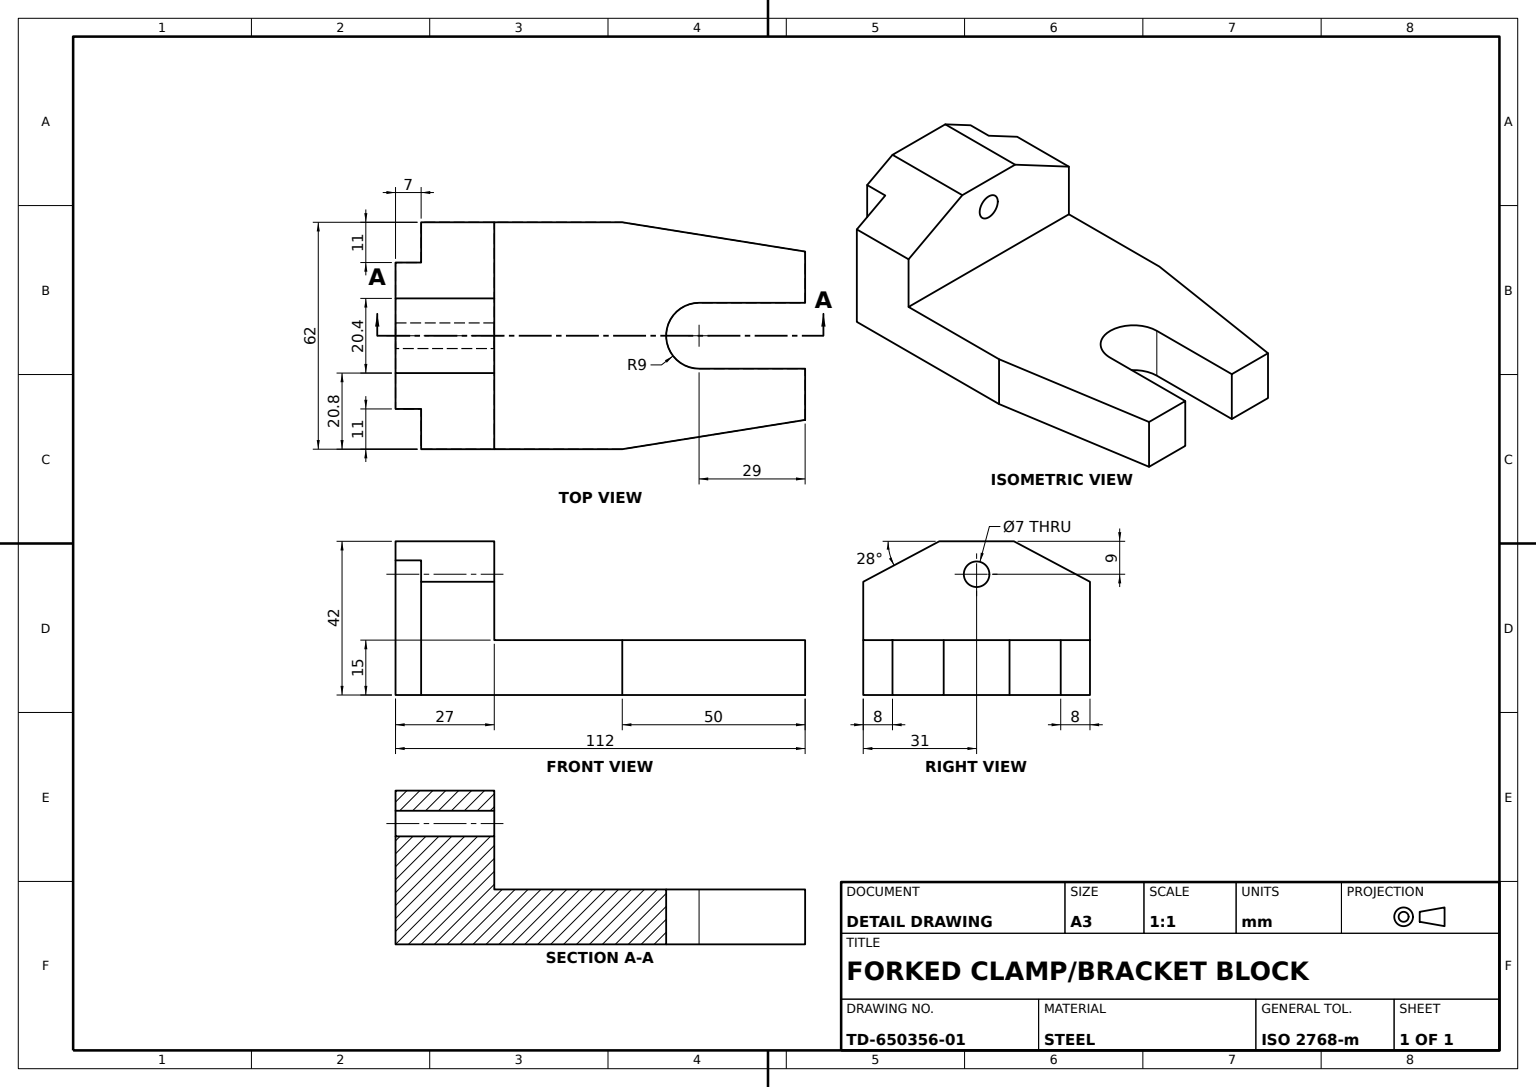
SolidWorks part; units mm, degrees
material "Plain Carbon Steel"
ref_plane "Front Plane" through (0, 0, 0) normal (0, 0, 1) x (1, 0, 0)
ref_plane "Top Plane" through (0, 0, 0) normal (0, 1, 0) x (1, 0, 0)
ref_plane "Right Plane" through (0, 0, 0) normal (1, 0, 0) x (0, 0, -1)
sketch "Bracket Profile Sketch" plane through (0, 0, 0) normal (0, 0, 1) x (1, 0, 0)
  line L1 (0, 0) -> (27, 0)
  line L2 (0, 0) -> (0, 42)
  line L3 (0, 42) -> (27, 42)
  line L4 (27, 15) -> (27, 42)
  line L5 (0, 0) -> (112, 0)
  line L6 (0, 0) -> (0, 15)
  line L7 (27, 15) -> (112, 15)
  line L8 (112, 0) -> (112, 15)
  dimension "D1" = 42
  dimension "D2" = 27
  dimension "D3" = 112
  dimension "D4" = 15
extrude "Bracket Body" add sketch "Bracket Profile Sketch" along normal mid plane 62 contours L5 L8 L7 L4 L3 L2 L1
sketch "Head Chamfer Sketch" plane through (27, 0, 0) normal (1, 0, 0) x (0, 0, -1)
  line L0 (10.203, 42) -> (31, 30.942)
  line L1 (-31, 42) -> (31, 42) construction
  line L2 (-10.2, 42) -> (-31, 30.9404)
  line L3 (31, 15) -> (31, 42) construction
  line L5 (-31, 30.9404) -> (-31, 54.9611)
  line L7 (-31, 54.9611) -> (31, 54.9611)
  line L8 (31, 54.9611) -> (31, 30.942)
  line L10 (-10.2, 42) -> (10.203, 42)
  circle A0 centre (0, 33) radius 3.5
  dimension "D4" = 7
  dimension "D1" = 28
  dimension "D2" = 28
  dimension "D3" = 9
  dimension "D5" = 20.403
  dimension "D6" = 10.2
  dimension "D7" = 20.797
  dimension "D8" = 62
  dimension "D9" = 12.9611
  dimension "D10" = 11.058
extrude "Head Chamfer Cut" cut sketch "Head Chamfer Sketch" against normal mid plane 62
sketch "Head Notch Sketch" plane through (0, 42, 0) normal (0, 1, 0) x (1, 0, 0)
  line L1 (0, 31) -> (7, 31)
  line L2 (0, 31) -> (0, 20)
  line L3 (0, 20) -> (7, 20)
  line L4 (7, 31) -> (7, 20)
  line L5 (0, -31) -> (7, -31)
  line L6 (0, -31) -> (0, -20)
  line L7 (0, -20) -> (7, -20)
  line L8 (7, -31) -> (7, -20)
  dimension "D1" = 11
  dimension "D2" = 7
  dimension "D3" = 11
  dimension "D4" = 7
extrude "Head Notch Cut" cut sketch "Head Notch Sketch" against normal mid plane 102
sketch "Forked Slot Sketch" plane through (0, 15, 0) normal (0, 1, 0) x (1, 0, 0)
  line L0 (62, -31) -> (112, -23)
  line L1 (27, -31) -> (112, -31) construction
  line L2 (62, 31) -> (112, 23)
  line L3 (27, 31) -> (112, 31) construction
  line L4 (83, 9) -> (112, 9)
  line L5 (83, -9) -> (112, -9)
  line L6 (112, 9) -> (112, -9)
  line L7 (62, 31) -> (112, 31)
  line L9 (62, -31) -> (112, -31)
  line L10 (112, 31) -> (112, 23)
  line L11 (112, -23) -> (112, -31)
  arc A0 (83, 9) -> (83, -9) centre (83, 0) ccw
  dimension "D1" = 18
  dimension "D2" = 29
  dimension "D3" = 50
  dimension "D4" = 50
  dimension "D5" = 8
  dimension "D6" = 8
extrude "Forked Slot Cut" cut sketch "Forked Slot Sketch" against normal blind 102
